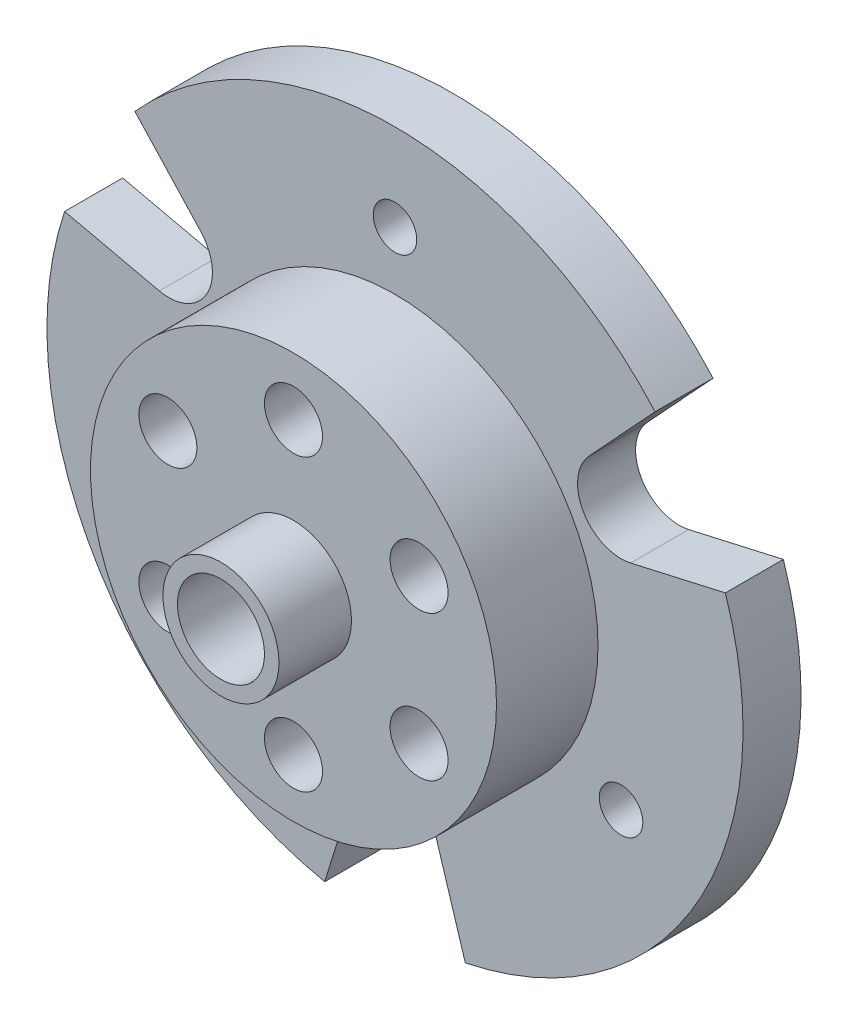
ISO-10303-21;
HEADER;
FILE_DESCRIPTION(('STEP AP214'),'2;1');
FILE_NAME('part.step','',(''),(''),'','','');
FILE_SCHEMA(('AUTOMOTIVE_DESIGN { 1 0 10303 214 1 1 1 1 }'));
ENDSEC;
DATA;
#1=APPLICATION_CONTEXT('core data for automotive mechanical design processes');
#2=APPLICATION_PROTOCOL_DEFINITION('international standard','automotive_design',2000,#1);
#3=PRODUCT_CONTEXT('',#1,'mechanical');
#4=PRODUCT('Part','Part','',(#3));
#5=PRODUCT_RELATED_PRODUCT_CATEGORY('part','',(#4));
#6=PRODUCT_DEFINITION_FORMATION('','',#4);
#7=PRODUCT_DEFINITION_CONTEXT('part definition',#1,'design');
#8=PRODUCT_DEFINITION('design','',#6,#7);
#9=PRODUCT_DEFINITION_SHAPE('','',#8);
#10=(LENGTH_UNIT() NAMED_UNIT(*) SI_UNIT(.MILLI.,.METRE.));
#11=(NAMED_UNIT(*) PLANE_ANGLE_UNIT() SI_UNIT($,.RADIAN.));
#12=(NAMED_UNIT(*) SI_UNIT($,.STERADIAN.) SOLID_ANGLE_UNIT());
#13=UNCERTAINTY_MEASURE_WITH_UNIT(LENGTH_MEASURE(1.E-05),#10,'distance_accuracy_value','');
#14=(GEOMETRIC_REPRESENTATION_CONTEXT(3) GLOBAL_UNCERTAINTY_ASSIGNED_CONTEXT((#13)) GLOBAL_UNIT_ASSIGNED_CONTEXT((#10,
#11,#12)) REPRESENTATION_CONTEXT('',''));
#15=CARTESIAN_POINT('',(0.,0.,0.));
#16=DIRECTION('',(0.,0.,1.));
#17=DIRECTION('',(1.,0.,0.));
#18=AXIS2_PLACEMENT_3D('',#15,#16,#17);
#19=CARTESIAN_POINT('',(0.,0.,4.));
#20=DIRECTION('',(0.,0.,-1.));
#21=DIRECTION('',(-1.,0.,0.));
#22=AXIS2_PLACEMENT_3D('',#19,#20,#21);
#23=CYLINDRICAL_SURFACE('',#22,24.);
#24=CARTESIAN_POINT('',(0.,0.,0.));
#25=DIRECTION('',(0.,0.,1.));
#26=DIRECTION('',(1.,0.,0.));
#27=AXIS2_PLACEMENT_3D('',#24,#25,#26);
#28=CIRCLE('',#27,24.);
#29=CARTESIAN_POINT('',(-22.7797497192924,7.5553294254054,0.));
#30=VERTEX_POINT('',#29);
#31=CARTESIAN_POINT('',(-4.84676764328516,-23.5055066614614,0.));
#32=VERTEX_POINT('',#31);
#33=EDGE_CURVE('E169',#30,#32,#28,.T.);
#34=ORIENTED_EDGE('',*,*,#33,.T.);
#35=DIRECTION('',(0.,0.,-1.));
#36=VECTOR('',#35,1.);
#37=CARTESIAN_POINT('',(-4.84676764328516,-23.5055066614614,4.));
#38=LINE('',#37,#36);
#39=CARTESIAN_POINT('',(-4.84676764328516,-23.5055066614614,4.));
#40=VERTEX_POINT('',#39);
#41=EDGE_CURVE('E53',#40,#32,#38,.T.);
#42=ORIENTED_EDGE('',*,*,#41,.F.);
#43=CARTESIAN_POINT('',(0.,0.,4.));
#44=DIRECTION('',(0.,0.,1.));
#45=DIRECTION('',(1.,0.,0.));
#46=AXIS2_PLACEMENT_3D('',#43,#44,#45);
#47=CIRCLE('',#46,24.);
#48=CARTESIAN_POINT('',(-22.7797497192924,7.5553294254054,4.));
#49=VERTEX_POINT('',#48);
#50=EDGE_CURVE('E191',#49,#40,#47,.T.);
#51=ORIENTED_EDGE('',*,*,#50,.F.);
#52=DIRECTION('',(0.,0.,-1.));
#53=VECTOR('',#52,1.);
#54=CARTESIAN_POINT('',(-22.7797497192924,7.5553294254054,4.));
#55=LINE('',#54,#53);
#56=EDGE_CURVE('E163',#49,#30,#55,.T.);
#57=ORIENTED_EDGE('',*,*,#56,.T.);
#58=EDGE_LOOP('',(#34,#42,#51,#57));
#59=FACE_BOUND('',#58,.T.);
#60=ADVANCED_FACE('F44',(#59),#23,.T.);
#61=CARTESIAN_POINT('',(-4.84676764328516,-23.5055066614614,4.));
#62=DIRECTION('',(-0.955190414845375,0.295992012371146,0.));
#63=DIRECTION('',(-0.295992012371146,-0.955190414845375,0.));
#64=AXIS2_PLACEMENT_3D('',#61,#62,#63);
#65=PLANE('',#64);
#66=DIRECTION('',(0.295992012371146,0.955190414845375,0.));
#67=VECTOR('',#66,1.);
#68=CARTESIAN_POINT('',(-4.84676764328516,-23.5055066614614,0.));
#69=LINE('',#68,#67);
#70=CARTESIAN_POINT('',(-2.86557124453613,-17.1120239628866,0.));
#71=VERTEX_POINT('',#70);
#72=EDGE_CURVE('E172',#32,#71,#69,.T.);
#73=ORIENTED_EDGE('',*,*,#72,.T.);
#74=DIRECTION('',(0.,0.,-1.));
#75=VECTOR('',#74,1.);
#76=CARTESIAN_POINT('',(-2.86557124453613,-17.1120239628866,4.));
#77=LINE('',#76,#75);
#78=CARTESIAN_POINT('',(-2.86557124453613,-17.1120239628866,4.));
#79=VERTEX_POINT('',#78);
#80=EDGE_CURVE('E213',#79,#71,#77,.T.);
#81=ORIENTED_EDGE('',*,*,#80,.F.);
#82=DIRECTION('',(0.295992012371146,0.955190414845375,0.));
#83=VECTOR('',#82,1.);
#84=CARTESIAN_POINT('',(-4.84676764328516,-23.5055066614614,4.));
#85=LINE('',#84,#83);
#86=EDGE_CURVE('E116',#40,#79,#85,.T.);
#87=ORIENTED_EDGE('',*,*,#86,.F.);
#88=ORIENTED_EDGE('',*,*,#41,.T.);
#89=EDGE_LOOP('',(#73,#81,#87,#88));
#90=FACE_BOUND('',#89,.T.);
#91=ADVANCED_FACE('F324',(#90),#65,.F.);
#92=CARTESIAN_POINT('',(0.,-18.,4.));
#93=DIRECTION('',(0.,0.,-1.));
#94=DIRECTION('',(-1.,0.,0.));
#95=AXIS2_PLACEMENT_3D('',#92,#93,#94);
#96=CYLINDRICAL_SURFACE('',#95,3.);
#97=CARTESIAN_POINT('',(0.,-18.,0.));
#98=DIRECTION('',(0.,0.,-1.));
#99=DIRECTION('',(1.,0.,0.));
#100=AXIS2_PLACEMENT_3D('',#97,#98,#99);
#101=CIRCLE('',#100,3.);
#102=CARTESIAN_POINT('',(2.86557124453613,-17.1120239628866,0.));
#103=VERTEX_POINT('',#102);
#104=EDGE_CURVE('E171',#71,#103,#101,.T.);
#105=ORIENTED_EDGE('',*,*,#104,.T.);
#106=DIRECTION('',(0.,0.,-1.));
#107=VECTOR('',#106,1.);
#108=CARTESIAN_POINT('',(2.86557124453613,-17.1120239628866,4.));
#109=LINE('',#108,#107);
#110=CARTESIAN_POINT('',(2.86557124453613,-17.1120239628866,4.));
#111=VERTEX_POINT('',#110);
#112=EDGE_CURVE('E209',#111,#103,#109,.T.);
#113=ORIENTED_EDGE('',*,*,#112,.F.);
#114=CARTESIAN_POINT('',(0.,-18.,4.));
#115=DIRECTION('',(0.,0.,-1.));
#116=DIRECTION('',(1.,0.,0.));
#117=AXIS2_PLACEMENT_3D('',#114,#115,#116);
#118=CIRCLE('',#117,3.);
#119=EDGE_CURVE('E283',#79,#111,#118,.T.);
#120=ORIENTED_EDGE('',*,*,#119,.F.);
#121=ORIENTED_EDGE('',*,*,#80,.T.);
#122=EDGE_LOOP('',(#105,#113,#120,#121));
#123=FACE_BOUND('',#122,.T.);
#124=ADVANCED_FACE('F328',(#123),#96,.F.);
#125=CARTESIAN_POINT('',(4.84676764328512,-23.5055066614614,4.));
#126=DIRECTION('',(0.955190414845377,0.29599201237114,0.));
#127=DIRECTION('',(-0.29599201237114,0.955190414845377,0.));
#128=AXIS2_PLACEMENT_3D('',#125,#126,#127);
#129=PLANE('',#128);
#130=DIRECTION('',(0.29599201237114,-0.955190414845377,0.));
#131=VECTOR('',#130,1.);
#132=CARTESIAN_POINT('',(4.84676764328512,-23.5055066614614,0.));
#133=LINE('',#132,#131);
#134=CARTESIAN_POINT('',(4.84676764328512,-23.5055066614614,0.));
#135=VERTEX_POINT('',#134);
#136=EDGE_CURVE('E176',#103,#135,#133,.T.);
#137=ORIENTED_EDGE('',*,*,#136,.T.);
#138=DIRECTION('',(0.,0.,-1.));
#139=VECTOR('',#138,1.);
#140=CARTESIAN_POINT('',(4.84676764328512,-23.5055066614614,4.));
#141=LINE('',#140,#139);
#142=CARTESIAN_POINT('',(4.84676764328512,-23.5055066614614,4.));
#143=VERTEX_POINT('',#142);
#144=EDGE_CURVE('E210',#143,#135,#141,.T.);
#145=ORIENTED_EDGE('',*,*,#144,.F.);
#146=DIRECTION('',(0.29599201237114,-0.955190414845377,0.));
#147=VECTOR('',#146,1.);
#148=CARTESIAN_POINT('',(4.84676764328512,-23.5055066614614,4.));
#149=LINE('',#148,#147);
#150=EDGE_CURVE('E290',#111,#143,#149,.T.);
#151=ORIENTED_EDGE('',*,*,#150,.F.);
#152=ORIENTED_EDGE('',*,*,#112,.T.);
#153=EDGE_LOOP('',(#137,#145,#151,#152));
#154=FACE_BOUND('',#153,.T.);
#155=ADVANCED_FACE('F334',(#154),#129,.F.);
#156=CARTESIAN_POINT('',(0.,0.,4.));
#157=DIRECTION('',(0.,0.,-1.));
#158=DIRECTION('',(-1.,0.,0.));
#159=AXIS2_PLACEMENT_3D('',#156,#157,#158);
#160=CYLINDRICAL_SURFACE('',#159,24.);
#161=CARTESIAN_POINT('',(0.,0.,0.));
#162=DIRECTION('',(0.,0.,1.));
#163=DIRECTION('',(1.,0.,0.));
#164=AXIS2_PLACEMENT_3D('',#161,#162,#163);
#165=CIRCLE('',#164,24.);
#166=CARTESIAN_POINT('',(22.7797497192925,7.55532942540507,0.));
#167=VERTEX_POINT('',#166);
#168=EDGE_CURVE('E177',#135,#167,#165,.T.);
#169=ORIENTED_EDGE('',*,*,#168,.T.);
#170=DIRECTION('',(0.,0.,-1.));
#171=VECTOR('',#170,1.);
#172=CARTESIAN_POINT('',(22.7797497192925,7.55532942540507,4.));
#173=LINE('',#172,#171);
#174=CARTESIAN_POINT('',(22.7797497192925,7.55532942540507,4.));
#175=VERTEX_POINT('',#174);
#176=EDGE_CURVE('E204',#175,#167,#173,.T.);
#177=ORIENTED_EDGE('',*,*,#176,.F.);
#178=CARTESIAN_POINT('',(0.,0.,4.));
#179=DIRECTION('',(0.,0.,1.));
#180=DIRECTION('',(1.,0.,0.));
#181=AXIS2_PLACEMENT_3D('',#178,#179,#180);
#182=CIRCLE('',#181,24.);
#183=EDGE_CURVE('E288',#143,#175,#182,.T.);
#184=ORIENTED_EDGE('',*,*,#183,.F.);
#185=ORIENTED_EDGE('',*,*,#144,.T.);
#186=EDGE_LOOP('',(#169,#177,#184,#185));
#187=FACE_BOUND('',#186,.T.);
#188=ADVANCED_FACE('F336',(#187),#160,.T.);
#189=CARTESIAN_POINT('',(22.7797497192925,7.55532942540508,4.));
#190=DIRECTION('',(0.221258605391988,-0.975215170893066,0.));
#191=DIRECTION('',(0.975215170893066,0.221258605391988,0.));
#192=AXIS2_PLACEMENT_3D('',#189,#190,#191);
#193=PLANE('',#192);
#194=DIRECTION('',(-0.975215170893066,-0.221258605391988,0.));
#195=VECTOR('',#194,1.);
#196=CARTESIAN_POINT('',(22.7797497192925,7.55532942540508,0.));
#197=LINE('',#196,#195);
#198=CARTESIAN_POINT('',(16.2522330842959,6.07435448732066,0.));
#199=VERTEX_POINT('',#198);
#200=EDGE_CURVE('E179',#167,#199,#197,.T.);
#201=ORIENTED_EDGE('',*,*,#200,.T.);
#202=DIRECTION('',(0.,0.,-1.));
#203=VECTOR('',#202,1.);
#204=CARTESIAN_POINT('',(16.2522330842959,6.07435448732066,4.));
#205=LINE('',#204,#203);
#206=CARTESIAN_POINT('',(16.2522330842959,6.07435448732066,4.));
#207=VERTEX_POINT('',#206);
#208=EDGE_CURVE('E203',#207,#199,#205,.T.);
#209=ORIENTED_EDGE('',*,*,#208,.F.);
#210=DIRECTION('',(-0.975215170893066,-0.221258605391988,0.));
#211=VECTOR('',#210,1.);
#212=CARTESIAN_POINT('',(22.7797497192925,7.55532942540508,4.));
#213=LINE('',#212,#211);
#214=EDGE_CURVE('E292',#175,#207,#213,.T.);
#215=ORIENTED_EDGE('',*,*,#214,.F.);
#216=ORIENTED_EDGE('',*,*,#176,.T.);
#217=EDGE_LOOP('',(#201,#209,#215,#216));
#218=FACE_BOUND('',#217,.T.);
#219=ADVANCED_FACE('F342',(#218),#193,.F.);
#220=CARTESIAN_POINT('',(15.58845726812,8.99999999999986,4.));
#221=DIRECTION('',(0.,0.,-1.));
#222=DIRECTION('',(-1.,0.,0.));
#223=AXIS2_PLACEMENT_3D('',#220,#221,#222);
#224=CYLINDRICAL_SURFACE('',#223,3.);
#225=CARTESIAN_POINT('',(15.58845726812,8.99999999999986,0.));
#226=DIRECTION('',(0.,0.,-1.));
#227=DIRECTION('',(1.,0.,0.));
#228=AXIS2_PLACEMENT_3D('',#225,#226,#227);
#229=CIRCLE('',#228,3.);
#230=CARTESIAN_POINT('',(13.3866618397599,11.0376694755656,0.));
#231=VERTEX_POINT('',#230);
#232=EDGE_CURVE('E185',#199,#231,#229,.T.);
#233=ORIENTED_EDGE('',*,*,#232,.T.);
#234=DIRECTION('',(0.,0.,-1.));
#235=VECTOR('',#234,1.);
#236=CARTESIAN_POINT('',(13.3866618397599,11.0376694755656,4.));
#237=LINE('',#236,#235);
#238=CARTESIAN_POINT('',(13.3866618397599,11.0376694755656,4.));
#239=VERTEX_POINT('',#238);
#240=EDGE_CURVE('E196',#239,#231,#237,.T.);
#241=ORIENTED_EDGE('',*,*,#240,.F.);
#242=CARTESIAN_POINT('',(15.58845726812,8.99999999999986,4.));
#243=DIRECTION('',(0.,0.,-1.));
#244=DIRECTION('',(1.,0.,0.));
#245=AXIS2_PLACEMENT_3D('',#242,#243,#244);
#246=CIRCLE('',#245,3.);
#247=EDGE_CURVE('E291',#207,#239,#246,.T.);
#248=ORIENTED_EDGE('',*,*,#247,.F.);
#249=ORIENTED_EDGE('',*,*,#208,.T.);
#250=EDGE_LOOP('',(#233,#241,#248,#249));
#251=FACE_BOUND('',#250,.T.);
#252=ADVANCED_FACE('F350',(#251),#224,.F.);
#253=CARTESIAN_POINT('',(17.9329820760075,15.9501772360559,4.));
#254=DIRECTION('',(-0.733931809453372,0.679223158521925,0.));
#255=DIRECTION('',(-0.679223158521925,-0.733931809453372,0.));
#256=AXIS2_PLACEMENT_3D('',#253,#254,#255);
#257=PLANE('',#256);
#258=DIRECTION('',(0.679223158521925,0.733931809453372,0.));
#259=VECTOR('',#258,1.);
#260=CARTESIAN_POINT('',(17.9329820760075,15.9501772360559,0.));
#261=LINE('',#260,#259);
#262=CARTESIAN_POINT('',(17.9329820760075,15.9501772360559,0.));
#263=VERTEX_POINT('',#262);
#264=EDGE_CURVE('E184',#231,#263,#261,.T.);
#265=ORIENTED_EDGE('',*,*,#264,.T.);
#266=DIRECTION('',(0.,0.,-1.));
#267=VECTOR('',#266,1.);
#268=CARTESIAN_POINT('',(17.9329820760075,15.9501772360559,4.));
#269=LINE('',#268,#267);
#270=CARTESIAN_POINT('',(17.9329820760075,15.9501772360559,4.));
#271=VERTEX_POINT('',#270);
#272=EDGE_CURVE('E194',#271,#263,#269,.T.);
#273=ORIENTED_EDGE('',*,*,#272,.F.);
#274=DIRECTION('',(0.679223158521925,0.733931809453372,0.));
#275=VECTOR('',#274,1.);
#276=CARTESIAN_POINT('',(17.9329820760075,15.9501772360559,4.));
#277=LINE('',#276,#275);
#278=EDGE_CURVE('E293',#239,#271,#277,.T.);
#279=ORIENTED_EDGE('',*,*,#278,.F.);
#280=ORIENTED_EDGE('',*,*,#240,.T.);
#281=EDGE_LOOP('',(#265,#273,#279,#280));
#282=FACE_BOUND('',#281,.T.);
#283=ADVANCED_FACE('F301',(#282),#257,.F.);
#284=CARTESIAN_POINT('',(0.,0.,4.));
#285=DIRECTION('',(0.,0.,-1.));
#286=DIRECTION('',(-1.,0.,0.));
#287=AXIS2_PLACEMENT_3D('',#284,#285,#286);
#288=CYLINDRICAL_SURFACE('',#287,24.);
#289=CARTESIAN_POINT('',(0.,0.,0.));
#290=DIRECTION('',(0.,0.,1.));
#291=DIRECTION('',(1.,0.,0.));
#292=AXIS2_PLACEMENT_3D('',#289,#290,#291);
#293=CIRCLE('',#292,24.);
#294=CARTESIAN_POINT('',(-17.9329820760072,15.9501772360561,0.));
#295=VERTEX_POINT('',#294);
#296=EDGE_CURVE('E187',#263,#295,#293,.T.);
#297=ORIENTED_EDGE('',*,*,#296,.T.);
#298=DIRECTION('',(0.,0.,-1.));
#299=VECTOR('',#298,1.);
#300=CARTESIAN_POINT('',(-17.9329820760072,15.9501772360561,4.));
#301=LINE('',#300,#299);
#302=CARTESIAN_POINT('',(-17.9329820760072,15.9501772360561,4.));
#303=VERTEX_POINT('',#302);
#304=EDGE_CURVE('E157',#303,#295,#301,.T.);
#305=ORIENTED_EDGE('',*,*,#304,.F.);
#306=CARTESIAN_POINT('',(0.,0.,4.));
#307=DIRECTION('',(0.,0.,1.));
#308=DIRECTION('',(1.,0.,0.));
#309=AXIS2_PLACEMENT_3D('',#306,#307,#308);
#310=CIRCLE('',#309,24.);
#311=EDGE_CURVE('E147',#271,#303,#310,.T.);
#312=ORIENTED_EDGE('',*,*,#311,.F.);
#313=ORIENTED_EDGE('',*,*,#272,.T.);
#314=EDGE_LOOP('',(#297,#305,#312,#313));
#315=FACE_BOUND('',#314,.T.);
#316=ADVANCED_FACE('F304',(#315),#288,.T.);
#317=CARTESIAN_POINT('',(-17.9329820760072,15.9501772360562,4.));
#318=DIRECTION('',(0.733931809453381,0.679223158521915,0.));
#319=DIRECTION('',(-0.679223158521915,0.733931809453381,0.));
#320=AXIS2_PLACEMENT_3D('',#317,#318,#319);
#321=PLANE('',#320);
#322=DIRECTION('',(0.679223158521915,-0.733931809453381,0.));
#323=VECTOR('',#322,1.);
#324=CARTESIAN_POINT('',(-17.9329820760072,15.9501772360562,0.));
#325=LINE('',#324,#323);
#326=CARTESIAN_POINT('',(-13.3866618397597,11.0376694755658,0.));
#327=VERTEX_POINT('',#326);
#328=EDGE_CURVE('E158',#295,#327,#325,.T.);
#329=ORIENTED_EDGE('',*,*,#328,.T.);
#330=DIRECTION('',(0.,0.,-1.));
#331=VECTOR('',#330,1.);
#332=CARTESIAN_POINT('',(-13.3866618397597,11.0376694755658,4.));
#333=LINE('',#332,#331);
#334=CARTESIAN_POINT('',(-13.3866618397597,11.0376694755658,4.));
#335=VERTEX_POINT('',#334);
#336=EDGE_CURVE('E154',#335,#327,#333,.T.);
#337=ORIENTED_EDGE('',*,*,#336,.F.);
#338=DIRECTION('',(0.679223158521915,-0.733931809453381,0.));
#339=VECTOR('',#338,1.);
#340=CARTESIAN_POINT('',(-17.9329820760072,15.9501772360562,4.));
#341=LINE('',#340,#339);
#342=EDGE_CURVE('E145',#303,#335,#341,.T.);
#343=ORIENTED_EDGE('',*,*,#342,.F.);
#344=ORIENTED_EDGE('',*,*,#304,.T.);
#345=EDGE_LOOP('',(#329,#337,#343,#344));
#346=FACE_BOUND('',#345,.T.);
#347=ADVANCED_FACE('F156',(#346),#321,.F.);
#348=CARTESIAN_POINT('',(-15.5884572681199,9.,4.));
#349=DIRECTION('',(0.,0.,-1.));
#350=DIRECTION('',(-1.,0.,0.));
#351=AXIS2_PLACEMENT_3D('',#348,#349,#350);
#352=CYLINDRICAL_SURFACE('',#351,3.);
#353=CARTESIAN_POINT('',(-15.5884572681199,9.,0.));
#354=DIRECTION('',(0.,0.,-1.));
#355=DIRECTION('',(1.,0.,0.));
#356=AXIS2_PLACEMENT_3D('',#353,#354,#355);
#357=CIRCLE('',#356,3.);
#358=CARTESIAN_POINT('',(-16.2522330842959,6.0743544873208,0.));
#359=VERTEX_POINT('',#358);
#360=EDGE_CURVE('E102',#327,#359,#357,.T.);
#361=ORIENTED_EDGE('',*,*,#360,.T.);
#362=DIRECTION('',(0.,0.,-1.));
#363=VECTOR('',#362,1.);
#364=CARTESIAN_POINT('',(-16.2522330842959,6.0743544873208,4.));
#365=LINE('',#364,#363);
#366=CARTESIAN_POINT('',(-16.2522330842959,6.0743544873208,4.));
#367=VERTEX_POINT('',#366);
#368=EDGE_CURVE('E159',#367,#359,#365,.T.);
#369=ORIENTED_EDGE('',*,*,#368,.F.);
#370=CARTESIAN_POINT('',(-15.5884572681199,9.,4.));
#371=DIRECTION('',(0.,0.,-1.));
#372=DIRECTION('',(1.,0.,0.));
#373=AXIS2_PLACEMENT_3D('',#370,#371,#372);
#374=CIRCLE('',#373,3.);
#375=EDGE_CURVE('E146',#335,#367,#374,.T.);
#376=ORIENTED_EDGE('',*,*,#375,.F.);
#377=ORIENTED_EDGE('',*,*,#336,.T.);
#378=EDGE_LOOP('',(#361,#369,#376,#377));
#379=FACE_BOUND('',#378,.T.);
#380=ADVANCED_FACE('F165',(#379),#352,.F.);
#381=CARTESIAN_POINT('',(-22.7797497192924,7.5553294254054,4.));
#382=DIRECTION('',(-0.221258605392001,-0.975215170893063,0.));
#383=DIRECTION('',(0.975215170893063,-0.221258605392001,0.));
#384=AXIS2_PLACEMENT_3D('',#381,#382,#383);
#385=PLANE('',#384);
#386=DIRECTION('',(-0.975215170893063,0.221258605392001,0.));
#387=VECTOR('',#386,1.);
#388=CARTESIAN_POINT('',(-22.7797497192924,7.5553294254054,0.));
#389=LINE('',#388,#387);
#390=EDGE_CURVE('E109',#359,#30,#389,.T.);
#391=ORIENTED_EDGE('',*,*,#390,.T.);
#392=ORIENTED_EDGE('',*,*,#56,.F.);
#393=DIRECTION('',(-0.975215170893063,0.221258605392001,0.));
#394=VECTOR('',#393,1.);
#395=CARTESIAN_POINT('',(-22.7797497192924,7.5553294254054,4.));
#396=LINE('',#395,#394);
#397=EDGE_CURVE('E65',#367,#49,#396,.T.);
#398=ORIENTED_EDGE('',*,*,#397,.F.);
#399=ORIENTED_EDGE('',*,*,#368,.T.);
#400=EDGE_LOOP('',(#391,#392,#398,#399));
#401=FACE_BOUND('',#400,.T.);
#402=ADVANCED_FACE('F311',(#401),#385,.F.);
#403=CARTESIAN_POINT('',(0.,0.,4.));
#404=DIRECTION('',(0.,0.,1.));
#405=DIRECTION('',(1.,0.,0.));
#406=AXIS2_PLACEMENT_3D('',#403,#404,#405);
#407=PLANE('',#406);
#408=CARTESIAN_POINT('',(0.,18.,4.));
#409=DIRECTION('',(0.,0.,1.));
#410=DIRECTION('',(1.,0.,0.));
#411=AXIS2_PLACEMENT_3D('',#408,#409,#410);
#412=CIRCLE('',#411,1.5);
#413=CARTESIAN_POINT('',(1.5,18.,4.));
#414=VERTEX_POINT('',#413);
#415=EDGE_CURVE('E219',#414,#414,#412,.T.);
#416=ORIENTED_EDGE('',*,*,#415,.F.);
#417=EDGE_LOOP('',(#416));
#418=FACE_BOUND('',#417,.T.);
#419=CARTESIAN_POINT('',(-15.5884572681187,-9.00000000000067,4.));
#420=DIRECTION('',(0.,0.,1.));
#421=DIRECTION('',(1.,0.,0.));
#422=AXIS2_PLACEMENT_3D('',#419,#420,#421);
#423=CIRCLE('',#422,1.50000000000146);
#424=CARTESIAN_POINT('',(-14.0884572681173,-9.00000000000067,4.));
#425=VERTEX_POINT('',#424);
#426=EDGE_CURVE('E735',#425,#425,#423,.T.);
#427=ORIENTED_EDGE('',*,*,#426,.F.);
#428=EDGE_LOOP('',(#427));
#429=FACE_BOUND('',#428,.T.);
#430=CARTESIAN_POINT('',(15.588457268121,-8.99999999999934,4.));
#431=DIRECTION('',(0.,0.,1.));
#432=DIRECTION('',(1.,0.,0.));
#433=AXIS2_PLACEMENT_3D('',#430,#431,#432);
#434=CIRCLE('',#433,1.50000000000099);
#435=CARTESIAN_POINT('',(17.088457268122,-8.99999999999934,4.));
#436=VERTEX_POINT('',#435);
#437=EDGE_CURVE('E240',#436,#436,#434,.T.);
#438=ORIENTED_EDGE('',*,*,#437,.F.);
#439=EDGE_LOOP('',(#438));
#440=FACE_BOUND('',#439,.T.);
#441=CARTESIAN_POINT('',(0.,0.,4.));
#442=DIRECTION('',(0.,0.,1.));
#443=DIRECTION('',(1.,0.,0.));
#444=AXIS2_PLACEMENT_3D('',#441,#442,#443);
#445=CIRCLE('',#444,14.);
#446=CARTESIAN_POINT('',(14.,0.,4.));
#447=VERTEX_POINT('',#446);
#448=EDGE_CURVE('E11',#447,#447,#445,.T.);
#449=ORIENTED_EDGE('',*,*,#448,.F.);
#450=EDGE_LOOP('',(#449));
#451=FACE_BOUND('',#450,.T.);
#452=ORIENTED_EDGE('',*,*,#50,.T.);
#453=ORIENTED_EDGE('',*,*,#86,.T.);
#454=ORIENTED_EDGE('',*,*,#119,.T.);
#455=ORIENTED_EDGE('',*,*,#150,.T.);
#456=ORIENTED_EDGE('',*,*,#183,.T.);
#457=ORIENTED_EDGE('',*,*,#214,.T.);
#458=ORIENTED_EDGE('',*,*,#247,.T.);
#459=ORIENTED_EDGE('',*,*,#278,.T.);
#460=ORIENTED_EDGE('',*,*,#311,.T.);
#461=ORIENTED_EDGE('',*,*,#342,.T.);
#462=ORIENTED_EDGE('',*,*,#375,.T.);
#463=ORIENTED_EDGE('',*,*,#397,.T.);
#464=EDGE_LOOP('',(#452,#453,#454,#455,#456,#457,#458,#459,#460,#461,#462,#463));
#465=FACE_BOUND('',#464,.T.);
#466=ADVANCED_FACE('F148',(#418,#429,#440,#451,#465),#407,.T.);
#467=CARTESIAN_POINT('',(0.,0.,0.));
#468=DIRECTION('',(0.,0.,1.));
#469=DIRECTION('',(1.,0.,0.));
#470=AXIS2_PLACEMENT_3D('',#467,#468,#469);
#471=PLANE('',#470);
#472=CARTESIAN_POINT('',(0.,18.,0.));
#473=DIRECTION('',(0.,0.,1.));
#474=DIRECTION('',(1.,0.,0.));
#475=AXIS2_PLACEMENT_3D('',#472,#473,#474);
#476=CIRCLE('',#475,1.5);
#477=CARTESIAN_POINT('',(1.5,18.,0.));
#478=VERTEX_POINT('',#477);
#479=EDGE_CURVE('E48',#478,#478,#476,.T.);
#480=ORIENTED_EDGE('',*,*,#479,.T.);
#481=EDGE_LOOP('',(#480));
#482=FACE_BOUND('',#481,.T.);
#483=CARTESIAN_POINT('',(-15.5884572681187,-9.00000000000067,0.));
#484=DIRECTION('',(0.,0.,1.));
#485=DIRECTION('',(1.,0.,0.));
#486=AXIS2_PLACEMENT_3D('',#483,#484,#485);
#487=CIRCLE('',#486,1.50000000000146);
#488=CARTESIAN_POINT('',(-14.0884572681173,-9.00000000000067,0.));
#489=VERTEX_POINT('',#488);
#490=EDGE_CURVE('E218',#489,#489,#487,.T.);
#491=ORIENTED_EDGE('',*,*,#490,.T.);
#492=EDGE_LOOP('',(#491));
#493=FACE_BOUND('',#492,.T.);
#494=CARTESIAN_POINT('',(15.588457268121,-8.99999999999934,0.));
#495=DIRECTION('',(0.,0.,1.));
#496=DIRECTION('',(1.,0.,0.));
#497=AXIS2_PLACEMENT_3D('',#494,#495,#496);
#498=CIRCLE('',#497,1.50000000000099);
#499=CARTESIAN_POINT('',(17.088457268122,-8.99999999999934,0.));
#500=VERTEX_POINT('',#499);
#501=EDGE_CURVE('E220',#500,#500,#498,.T.);
#502=ORIENTED_EDGE('',*,*,#501,.T.);
#503=EDGE_LOOP('',(#502));
#504=FACE_BOUND('',#503,.T.);
#505=CARTESIAN_POINT('',(0.,0.,0.));
#506=DIRECTION('',(0.,0.,1.));
#507=DIRECTION('',(1.,0.,0.));
#508=AXIS2_PLACEMENT_3D('',#505,#506,#507);
#509=CIRCLE('',#508,3.);
#510=CARTESIAN_POINT('',(3.,0.,0.));
#511=VERTEX_POINT('',#510);
#512=EDGE_CURVE('E226',#511,#511,#509,.T.);
#513=ORIENTED_EDGE('',*,*,#512,.T.);
#514=EDGE_LOOP('',(#513));
#515=FACE_BOUND('',#514,.T.);
#516=CARTESIAN_POINT('',(0.,10.,0.));
#517=DIRECTION('',(0.,0.,1.));
#518=DIRECTION('',(1.,0.,0.));
#519=AXIS2_PLACEMENT_3D('',#516,#517,#518);
#520=CIRCLE('',#519,2.);
#521=CARTESIAN_POINT('',(2.,10.,0.));
#522=VERTEX_POINT('',#521);
#523=EDGE_CURVE('E279',#522,#522,#520,.T.);
#524=ORIENTED_EDGE('',*,*,#523,.T.);
#525=EDGE_LOOP('',(#524));
#526=FACE_BOUND('',#525,.T.);
#527=CARTESIAN_POINT('',(8.6602540378446,5.00000000000037,0.));
#528=DIRECTION('',(0.,0.,1.));
#529=DIRECTION('',(1.,0.,0.));
#530=AXIS2_PLACEMENT_3D('',#527,#528,#529);
#531=CIRCLE('',#530,2.00000000000012);
#532=CARTESIAN_POINT('',(10.6602540378447,5.00000000000037,0.));
#533=VERTEX_POINT('',#532);
#534=EDGE_CURVE('E274',#533,#533,#531,.T.);
#535=ORIENTED_EDGE('',*,*,#534,.T.);
#536=EDGE_LOOP('',(#535));
#537=FACE_BOUND('',#536,.T.);
#538=CARTESIAN_POINT('',(8.66025403784502,-4.99999999999963,0.));
#539=DIRECTION('',(0.,0.,1.));
#540=DIRECTION('',(1.,0.,0.));
#541=AXIS2_PLACEMENT_3D('',#538,#539,#540);
#542=CIRCLE('',#541,2.00000000000055);
#543=CARTESIAN_POINT('',(10.6602540378456,-4.99999999999963,0.));
#544=VERTEX_POINT('',#543);
#545=EDGE_CURVE('E275',#544,#544,#542,.T.);
#546=ORIENTED_EDGE('',*,*,#545,.T.);
#547=EDGE_LOOP('',(#546));
#548=FACE_BOUND('',#547,.T.);
#549=CARTESIAN_POINT('',(8.48977342514678E-13,-10.,0.));
#550=DIRECTION('',(0.,0.,1.));
#551=DIRECTION('',(1.,0.,0.));
#552=AXIS2_PLACEMENT_3D('',#549,#550,#551);
#553=CIRCLE('',#552,2.00000000000088);
#554=CARTESIAN_POINT('',(2.00000000000173,-10.,0.));
#555=VERTEX_POINT('',#554);
#556=EDGE_CURVE('E267',#555,#555,#553,.T.);
#557=ORIENTED_EDGE('',*,*,#556,.T.);
#558=EDGE_LOOP('',(#557));
#559=FACE_BOUND('',#558,.T.);
#560=CARTESIAN_POINT('',(-8.66025403784375,-5.00000000000037,0.));
#561=DIRECTION('',(0.,0.,1.));
#562=DIRECTION('',(1.,0.,0.));
#563=AXIS2_PLACEMENT_3D('',#560,#561,#562);
#564=CIRCLE('',#563,2.00000000000081);
#565=CARTESIAN_POINT('',(-6.66025403784294,-5.00000000000037,0.));
#566=VERTEX_POINT('',#565);
#567=EDGE_CURVE('E266',#566,#566,#564,.T.);
#568=ORIENTED_EDGE('',*,*,#567,.T.);
#569=EDGE_LOOP('',(#568));
#570=FACE_BOUND('',#569,.T.);
#571=CARTESIAN_POINT('',(-8.66025403784418,4.99999999999963,0.));
#572=DIRECTION('',(0.,0.,1.));
#573=DIRECTION('',(1.,0.,0.));
#574=AXIS2_PLACEMENT_3D('',#571,#572,#573);
#575=CIRCLE('',#574,2.00000000000043);
#576=CARTESIAN_POINT('',(-6.66025403784375,4.99999999999963,0.));
#577=VERTEX_POINT('',#576);
#578=EDGE_CURVE('E263',#577,#577,#575,.T.);
#579=ORIENTED_EDGE('',*,*,#578,.T.);
#580=EDGE_LOOP('',(#579));
#581=FACE_BOUND('',#580,.T.);
#582=ORIENTED_EDGE('',*,*,#33,.F.);
#583=ORIENTED_EDGE('',*,*,#390,.F.);
#584=ORIENTED_EDGE('',*,*,#360,.F.);
#585=ORIENTED_EDGE('',*,*,#328,.F.);
#586=ORIENTED_EDGE('',*,*,#296,.F.);
#587=ORIENTED_EDGE('',*,*,#264,.F.);
#588=ORIENTED_EDGE('',*,*,#232,.F.);
#589=ORIENTED_EDGE('',*,*,#200,.F.);
#590=ORIENTED_EDGE('',*,*,#168,.F.);
#591=ORIENTED_EDGE('',*,*,#136,.F.);
#592=ORIENTED_EDGE('',*,*,#104,.F.);
#593=ORIENTED_EDGE('',*,*,#72,.F.);
#594=EDGE_LOOP('',(#582,#583,#584,#585,#586,#587,#588,#589,#590,#591,#592,#593));
#595=FACE_BOUND('',#594,.T.);
#596=ADVANCED_FACE('F306',(#482,#493,#504,#515,#526,#537,#548,#559,#570,#581,#595),#471,.F.);
#597=CARTESIAN_POINT('',(0.,0.,11.));
#598=DIRECTION('',(0.,0.,-1.));
#599=DIRECTION('',(-1.,0.,0.));
#600=AXIS2_PLACEMENT_3D('',#597,#598,#599);
#601=CYLINDRICAL_SURFACE('',#600,14.);
#602=CARTESIAN_POINT('',(0.,0.,11.));
#603=DIRECTION('',(0.,0.,1.));
#604=DIRECTION('',(1.,0.,0.));
#605=AXIS2_PLACEMENT_3D('',#602,#603,#604);
#606=CIRCLE('',#605,14.);
#607=CARTESIAN_POINT('',(14.,0.,11.));
#608=VERTEX_POINT('',#607);
#609=EDGE_CURVE('E174',#608,#608,#606,.T.);
#610=ORIENTED_EDGE('',*,*,#609,.F.);
#611=EDGE_LOOP('',(#610));
#612=FACE_BOUND('',#611,.T.);
#613=ORIENTED_EDGE('',*,*,#448,.T.);
#614=EDGE_LOOP('',(#613));
#615=FACE_BOUND('',#614,.T.);
#616=ADVANCED_FACE('F387',(#612,#615),#601,.T.);
#617=CARTESIAN_POINT('',(0.,0.,11.));
#618=DIRECTION('',(0.,0.,1.));
#619=DIRECTION('',(1.,0.,0.));
#620=AXIS2_PLACEMENT_3D('',#617,#618,#619);
#621=PLANE('',#620);
#622=CARTESIAN_POINT('',(0.,0.,11.));
#623=DIRECTION('',(0.,0.,1.));
#624=DIRECTION('',(1.,0.,0.));
#625=AXIS2_PLACEMENT_3D('',#622,#623,#624);
#626=CIRCLE('',#625,4.);
#627=CARTESIAN_POINT('',(4.,0.,11.));
#628=VERTEX_POINT('',#627);
#629=EDGE_CURVE('E233',#628,#628,#626,.T.);
#630=ORIENTED_EDGE('',*,*,#629,.F.);
#631=EDGE_LOOP('',(#630));
#632=FACE_BOUND('',#631,.T.);
#633=CARTESIAN_POINT('',(0.,10.,11.));
#634=DIRECTION('',(0.,0.,1.));
#635=DIRECTION('',(1.,0.,0.));
#636=AXIS2_PLACEMENT_3D('',#633,#634,#635);
#637=CIRCLE('',#636,2.);
#638=CARTESIAN_POINT('',(2.,10.,11.));
#639=VERTEX_POINT('',#638);
#640=EDGE_CURVE('E245',#639,#639,#637,.T.);
#641=ORIENTED_EDGE('',*,*,#640,.F.);
#642=EDGE_LOOP('',(#641));
#643=FACE_BOUND('',#642,.T.);
#644=CARTESIAN_POINT('',(8.6602540378446,5.00000000000037,11.));
#645=DIRECTION('',(0.,0.,1.));
#646=DIRECTION('',(1.,0.,0.));
#647=AXIS2_PLACEMENT_3D('',#644,#645,#646);
#648=CIRCLE('',#647,2.00000000000012);
#649=CARTESIAN_POINT('',(10.6602540378447,5.00000000000037,11.));
#650=VERTEX_POINT('',#649);
#651=EDGE_CURVE('E258',#650,#650,#648,.T.);
#652=ORIENTED_EDGE('',*,*,#651,.F.);
#653=EDGE_LOOP('',(#652));
#654=FACE_BOUND('',#653,.T.);
#655=CARTESIAN_POINT('',(8.66025403784502,-4.99999999999963,11.));
#656=DIRECTION('',(0.,0.,1.));
#657=DIRECTION('',(1.,0.,0.));
#658=AXIS2_PLACEMENT_3D('',#655,#656,#657);
#659=CIRCLE('',#658,2.00000000000055);
#660=CARTESIAN_POINT('',(10.6602540378456,-4.99999999999963,11.));
#661=VERTEX_POINT('',#660);
#662=EDGE_CURVE('E251',#661,#661,#659,.T.);
#663=ORIENTED_EDGE('',*,*,#662,.F.);
#664=EDGE_LOOP('',(#663));
#665=FACE_BOUND('',#664,.T.);
#666=CARTESIAN_POINT('',(8.48977342514678E-13,-10.,11.));
#667=DIRECTION('',(0.,0.,1.));
#668=DIRECTION('',(1.,0.,0.));
#669=AXIS2_PLACEMENT_3D('',#666,#667,#668);
#670=CIRCLE('',#669,2.00000000000088);
#671=CARTESIAN_POINT('',(2.00000000000173,-10.,11.));
#672=VERTEX_POINT('',#671);
#673=EDGE_CURVE('E249',#672,#672,#670,.T.);
#674=ORIENTED_EDGE('',*,*,#673,.F.);
#675=EDGE_LOOP('',(#674));
#676=FACE_BOUND('',#675,.T.);
#677=CARTESIAN_POINT('',(-8.66025403784375,-5.00000000000037,11.));
#678=DIRECTION('',(0.,0.,1.));
#679=DIRECTION('',(1.,0.,0.));
#680=AXIS2_PLACEMENT_3D('',#677,#678,#679);
#681=CIRCLE('',#680,2.00000000000081);
#682=CARTESIAN_POINT('',(-6.66025403784294,-5.00000000000037,11.));
#683=VERTEX_POINT('',#682);
#684=EDGE_CURVE('E246',#683,#683,#681,.T.);
#685=ORIENTED_EDGE('',*,*,#684,.F.);
#686=EDGE_LOOP('',(#685));
#687=FACE_BOUND('',#686,.T.);
#688=CARTESIAN_POINT('',(-8.66025403784418,4.99999999999963,11.));
#689=DIRECTION('',(0.,0.,1.));
#690=DIRECTION('',(1.,0.,0.));
#691=AXIS2_PLACEMENT_3D('',#688,#689,#690);
#692=CIRCLE('',#691,2.00000000000043);
#693=CARTESIAN_POINT('',(-6.66025403784375,4.99999999999963,11.));
#694=VERTEX_POINT('',#693);
#695=EDGE_CURVE('E248',#694,#694,#692,.T.);
#696=ORIENTED_EDGE('',*,*,#695,.F.);
#697=EDGE_LOOP('',(#696));
#698=FACE_BOUND('',#697,.T.);
#699=ORIENTED_EDGE('',*,*,#609,.T.);
#700=EDGE_LOOP('',(#699));
#701=FACE_BOUND('',#700,.T.);
#702=ADVANCED_FACE('F400',(#632,#643,#654,#665,#676,#687,#698,#701),#621,.T.);
#703=CARTESIAN_POINT('',(-8.66025403784418,4.99999999999963,-19.));
#704=DIRECTION('',(0.,0.,1.));
#705=DIRECTION('',(1.,0.,0.));
#706=AXIS2_PLACEMENT_3D('',#703,#704,#705);
#707=CYLINDRICAL_SURFACE('',#706,2.00000000000043);
#708=ORIENTED_EDGE('',*,*,#695,.T.);
#709=EDGE_LOOP('',(#708));
#710=FACE_BOUND('',#709,.T.);
#711=ORIENTED_EDGE('',*,*,#578,.F.);
#712=EDGE_LOOP('',(#711));
#713=FACE_BOUND('',#712,.T.);
#714=ADVANCED_FACE('F394',(#710,#713),#707,.F.);
#715=CARTESIAN_POINT('',(-8.66025403784375,-5.00000000000037,-19.));
#716=DIRECTION('',(0.,0.,1.));
#717=DIRECTION('',(1.,0.,0.));
#718=AXIS2_PLACEMENT_3D('',#715,#716,#717);
#719=CYLINDRICAL_SURFACE('',#718,2.00000000000081);
#720=ORIENTED_EDGE('',*,*,#684,.T.);
#721=EDGE_LOOP('',(#720));
#722=FACE_BOUND('',#721,.T.);
#723=ORIENTED_EDGE('',*,*,#567,.F.);
#724=EDGE_LOOP('',(#723));
#725=FACE_BOUND('',#724,.T.);
#726=ADVANCED_FACE('F396',(#722,#725),#719,.F.);
#727=CARTESIAN_POINT('',(8.48977342514678E-13,-10.,-19.));
#728=DIRECTION('',(0.,0.,1.));
#729=DIRECTION('',(1.,0.,0.));
#730=AXIS2_PLACEMENT_3D('',#727,#728,#729);
#731=CYLINDRICAL_SURFACE('',#730,2.00000000000088);
#732=ORIENTED_EDGE('',*,*,#673,.T.);
#733=EDGE_LOOP('',(#732));
#734=FACE_BOUND('',#733,.T.);
#735=ORIENTED_EDGE('',*,*,#556,.F.);
#736=EDGE_LOOP('',(#735));
#737=FACE_BOUND('',#736,.T.);
#738=ADVANCED_FACE('F409',(#734,#737),#731,.F.);
#739=CARTESIAN_POINT('',(8.66025403784502,-4.99999999999963,-19.));
#740=DIRECTION('',(0.,0.,1.));
#741=DIRECTION('',(1.,0.,0.));
#742=AXIS2_PLACEMENT_3D('',#739,#740,#741);
#743=CYLINDRICAL_SURFACE('',#742,2.00000000000055);
#744=ORIENTED_EDGE('',*,*,#662,.T.);
#745=EDGE_LOOP('',(#744));
#746=FACE_BOUND('',#745,.T.);
#747=ORIENTED_EDGE('',*,*,#545,.F.);
#748=EDGE_LOOP('',(#747));
#749=FACE_BOUND('',#748,.T.);
#750=ADVANCED_FACE('F417',(#746,#749),#743,.F.);
#751=CARTESIAN_POINT('',(8.6602540378446,5.00000000000037,-19.));
#752=DIRECTION('',(0.,0.,1.));
#753=DIRECTION('',(1.,0.,0.));
#754=AXIS2_PLACEMENT_3D('',#751,#752,#753);
#755=CYLINDRICAL_SURFACE('',#754,2.00000000000012);
#756=ORIENTED_EDGE('',*,*,#651,.T.);
#757=EDGE_LOOP('',(#756));
#758=FACE_BOUND('',#757,.T.);
#759=ORIENTED_EDGE('',*,*,#534,.F.);
#760=EDGE_LOOP('',(#759));
#761=FACE_BOUND('',#760,.T.);
#762=ADVANCED_FACE('F430',(#758,#761),#755,.F.);
#763=CARTESIAN_POINT('',(0.,10.,-19.));
#764=DIRECTION('',(0.,0.,1.));
#765=DIRECTION('',(1.,0.,0.));
#766=AXIS2_PLACEMENT_3D('',#763,#764,#765);
#767=CYLINDRICAL_SURFACE('',#766,2.);
#768=ORIENTED_EDGE('',*,*,#640,.T.);
#769=EDGE_LOOP('',(#768));
#770=FACE_BOUND('',#769,.T.);
#771=ORIENTED_EDGE('',*,*,#523,.F.);
#772=EDGE_LOOP('',(#771));
#773=FACE_BOUND('',#772,.T.);
#774=ADVANCED_FACE('F440',(#770,#773),#767,.F.);
#775=CARTESIAN_POINT('',(0.,0.,16.));
#776=DIRECTION('',(0.,0.,-1.));
#777=DIRECTION('',(-1.,0.,0.));
#778=AXIS2_PLACEMENT_3D('',#775,#776,#777);
#779=CYLINDRICAL_SURFACE('',#778,4.);
#780=CARTESIAN_POINT('',(0.,0.,16.));
#781=DIRECTION('',(0.,0.,1.));
#782=DIRECTION('',(1.,0.,0.));
#783=AXIS2_PLACEMENT_3D('',#780,#781,#782);
#784=CIRCLE('',#783,4.);
#785=CARTESIAN_POINT('',(4.,0.,16.));
#786=VERTEX_POINT('',#785);
#787=EDGE_CURVE('E238',#786,#786,#784,.T.);
#788=ORIENTED_EDGE('',*,*,#787,.F.);
#789=EDGE_LOOP('',(#788));
#790=FACE_BOUND('',#789,.T.);
#791=ORIENTED_EDGE('',*,*,#629,.T.);
#792=EDGE_LOOP('',(#791));
#793=FACE_BOUND('',#792,.T.);
#794=ADVANCED_FACE('F449',(#790,#793),#779,.T.);
#795=CARTESIAN_POINT('',(0.,0.,16.));
#796=DIRECTION('',(0.,0.,1.));
#797=DIRECTION('',(1.,0.,0.));
#798=AXIS2_PLACEMENT_3D('',#795,#796,#797);
#799=PLANE('',#798);
#800=CARTESIAN_POINT('',(0.,0.,16.));
#801=DIRECTION('',(0.,0.,1.));
#802=DIRECTION('',(1.,0.,0.));
#803=AXIS2_PLACEMENT_3D('',#800,#801,#802);
#804=CIRCLE('',#803,3.);
#805=CARTESIAN_POINT('',(3.,0.,16.));
#806=VERTEX_POINT('',#805);
#807=EDGE_CURVE('E223',#806,#806,#804,.T.);
#808=ORIENTED_EDGE('',*,*,#807,.F.);
#809=EDGE_LOOP('',(#808));
#810=FACE_BOUND('',#809,.T.);
#811=ORIENTED_EDGE('',*,*,#787,.T.);
#812=EDGE_LOOP('',(#811));
#813=FACE_BOUND('',#812,.T.);
#814=ADVANCED_FACE('F498',(#810,#813),#799,.T.);
#815=CARTESIAN_POINT('',(0.,0.,-34.));
#816=DIRECTION('',(0.,0.,1.));
#817=DIRECTION('',(1.,0.,0.));
#818=AXIS2_PLACEMENT_3D('',#815,#816,#817);
#819=CYLINDRICAL_SURFACE('',#818,3.);
#820=ORIENTED_EDGE('',*,*,#807,.T.);
#821=EDGE_LOOP('',(#820));
#822=FACE_BOUND('',#821,.T.);
#823=ORIENTED_EDGE('',*,*,#512,.F.);
#824=EDGE_LOOP('',(#823));
#825=FACE_BOUND('',#824,.T.);
#826=ADVANCED_FACE('F459',(#822,#825),#819,.F.);
#827=CARTESIAN_POINT('',(15.588457268121,-8.99999999999934,-26.));
#828=DIRECTION('',(0.,0.,1.));
#829=DIRECTION('',(1.,0.,0.));
#830=AXIS2_PLACEMENT_3D('',#827,#828,#829);
#831=CYLINDRICAL_SURFACE('',#830,1.50000000000099);
#832=ORIENTED_EDGE('',*,*,#437,.T.);
#833=EDGE_LOOP('',(#832));
#834=FACE_BOUND('',#833,.T.);
#835=ORIENTED_EDGE('',*,*,#501,.F.);
#836=EDGE_LOOP('',(#835));
#837=FACE_BOUND('',#836,.T.);
#838=ADVANCED_FACE('F454',(#834,#837),#831,.F.);
#839=CARTESIAN_POINT('',(-15.5884572681187,-9.00000000000067,-26.));
#840=DIRECTION('',(0.,0.,1.));
#841=DIRECTION('',(1.,0.,0.));
#842=AXIS2_PLACEMENT_3D('',#839,#840,#841);
#843=CYLINDRICAL_SURFACE('',#842,1.50000000000146);
#844=ORIENTED_EDGE('',*,*,#426,.T.);
#845=EDGE_LOOP('',(#844));
#846=FACE_BOUND('',#845,.T.);
#847=ORIENTED_EDGE('',*,*,#490,.F.);
#848=EDGE_LOOP('',(#847));
#849=FACE_BOUND('',#848,.T.);
#850=ADVANCED_FACE('F456',(#846,#849),#843,.F.);
#851=CARTESIAN_POINT('',(0.,18.,-26.));
#852=DIRECTION('',(0.,0.,1.));
#853=DIRECTION('',(1.,0.,0.));
#854=AXIS2_PLACEMENT_3D('',#851,#852,#853);
#855=CYLINDRICAL_SURFACE('',#854,1.5);
#856=ORIENTED_EDGE('',*,*,#415,.T.);
#857=EDGE_LOOP('',(#856));
#858=FACE_BOUND('',#857,.T.);
#859=ORIENTED_EDGE('',*,*,#479,.F.);
#860=EDGE_LOOP('',(#859));
#861=FACE_BOUND('',#860,.T.);
#862=ADVANCED_FACE('F468',(#858,#861),#855,.F.);
#863=CLOSED_SHELL('',(#60,#91,#124,#155,#188,#219,#252,#283,#316,#347,#380,#402,#466,#596,#616,
#702,#714,#726,#738,#750,#762,#774,#794,#814,#826,#838,#850,#862));
#864=MANIFOLD_SOLID_BREP('B2',#863);
#865=ADVANCED_BREP_SHAPE_REPRESENTATION('',(#18,#864),#14);
#866=SHAPE_DEFINITION_REPRESENTATION(#9,#865);
ENDSEC;
END-ISO-10303-21;
